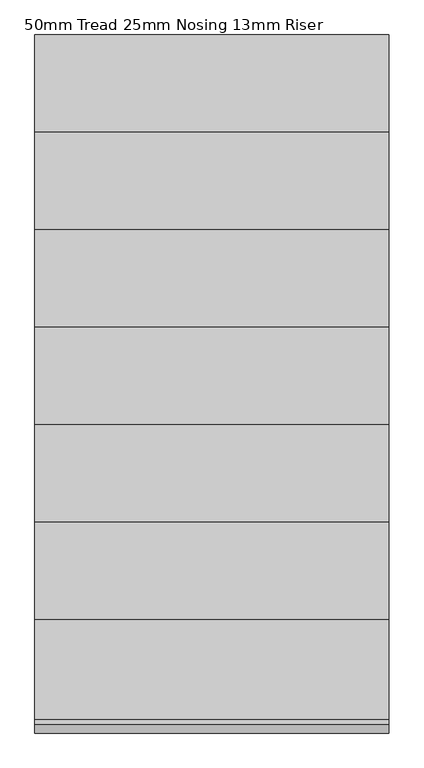
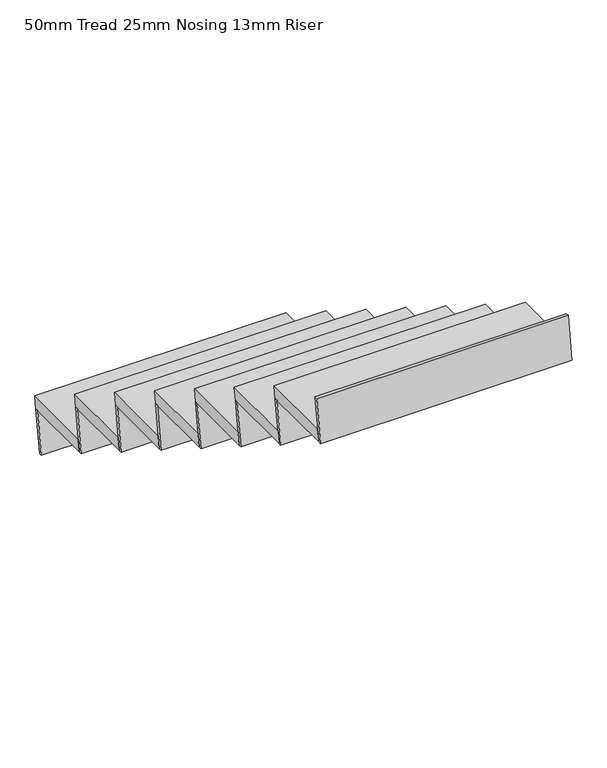
"""IFC4 building model written with IfcOpenShell, lengths in millimetres: stair flight geometry, 50mm Tread 25mm Nosing 13mm Riser."""

from ifc_helpers import new_model, si_unit, frame, origin, place, context, project, spatial, polyline, outline, extrude, source, transform, mapped, element, save


def stair_flight_50mm_tread_25mm_nosing_13mm_riser_d224a7c8(model_context):
    return source(origin(), model_context, "Body", "SweptSolid", [
        extrude(outline(polyline([(9522.57664, 869.5652174), (9822.57664, 869.5652174), (9815.38914, 819.5652174), (9515.38914, 819.5652174), (9522.57664, 869.5652174)])), frame((-8867.5141631, 0.0, 0.0), z_axis=(1.0, 0.0, 0.0), x_axis=(0.0, 1.0, 0.0)), (0.0, 0.0, 1.0), 1000.0257812),
        extrude(outline(polyline([(9815.38914, 819.5652174), (9790.38914, 645.6521739), (9777.76065, 645.6521739), (9802.76065, 819.5652174), (9815.38914, 819.5652174)])), frame((-8867.5141631, 0.0, 0.0), z_axis=(1.0, 0.0, 0.0), x_axis=(0.0, 1.0, 0.0)), (0.0, 0.0, 1.0), 1000.0257812),
        extrude(outline(polyline([(9540.38914, 993.4782609), (9515.38914, 819.5652174), (9502.76065, 819.5652174), (9527.76065, 993.4782609), (9540.38914, 993.4782609)])), frame((-8867.5141631, 0.0, 0.0), z_axis=(1.0, 0.0, 0.0), x_axis=(0.0, 1.0, 0.0)), (0.0, 0.0, 1.0), 1000.0257812),
        extrude(outline(polyline([(9247.57664, 1043.4782609), (9547.57664, 1043.4782609), (9540.38914, 993.4782609), (9240.38914, 993.4782609), (9247.57664, 1043.4782609)])), frame((-8867.5141631, 0.0, 0.0), z_axis=(1.0, 0.0, 0.0), x_axis=(0.0, 1.0, 0.0)), (0.0, 0.0, 1.0), 1000.0257812),
        extrude(outline(polyline([(9265.38914, 1167.3913043), (9240.38914, 993.4782609), (9227.76065, 993.4782609), (9252.76065, 1167.3913043), (9265.38914, 1167.3913043)])), frame((-8867.5141631, 0.0, 0.0), z_axis=(1.0, 0.0, 0.0), x_axis=(0.0, 1.0, 0.0)), (0.0, 0.0, 1.0), 1000.0257812),
        extrude(outline(polyline([(8972.57664, 1217.3913043), (9272.57664, 1217.3913043), (9265.38914, 1167.3913043), (8965.38914, 1167.3913043), (8972.57664, 1217.3913043)])), frame((-8867.5141631, 0.0, 0.0), z_axis=(1.0, 0.0, 0.0), x_axis=(0.0, 1.0, 0.0)), (0.0, 0.0, 1.0), 1000.0257812),
        extrude(outline(polyline([(8990.38914, 1341.3043478), (8965.38914, 1167.3913043), (8952.76065, 1167.3913043), (8977.76065, 1341.3043478), (8990.38914, 1341.3043478)])), frame((-8867.5141631, 0.0, 0.0), z_axis=(1.0, 0.0, 0.0), x_axis=(0.0, 1.0, 0.0)), (0.0, 0.0, 1.0), 1000.0257812),
        extrude(outline(polyline([(8697.57664, 1391.3043478), (8997.57664, 1391.3043478), (8990.38914, 1341.3043478), (8690.38914, 1341.3043478), (8697.57664, 1391.3043478)])), frame((-8867.5141631, 0.0, 0.0), z_axis=(1.0, 0.0, 0.0), x_axis=(0.0, 1.0, 0.0)), (0.0, 0.0, 1.0), 1000.0257812),
        extrude(outline(polyline([(8715.38914, 1515.2173913), (8690.38914, 1341.3043478), (8677.76065, 1341.3043478), (8702.76065, 1515.2173913), (8715.38914, 1515.2173913)])), frame((-8867.5141631, 0.0, 0.0), z_axis=(1.0, 0.0, 0.0), x_axis=(0.0, 1.0, 0.0)), (0.0, 0.0, 1.0), 1000.0257812),
        extrude(outline(polyline([(8422.57664, 1565.2173913), (8722.57664, 1565.2173913), (8715.38914, 1515.2173913), (8415.38914, 1515.2173913), (8422.57664, 1565.2173913)])), frame((-8867.5141631, 0.0, 0.0), z_axis=(1.0, 0.0, 0.0), x_axis=(0.0, 1.0, 0.0)), (0.0, 0.0, 1.0), 1000.0257812),
        extrude(outline(polyline([(8440.38914, 1689.1304348), (8415.38914, 1515.2173913), (8402.76065, 1515.2173913), (8427.76065, 1689.1304348), (8440.38914, 1689.1304348)])), frame((-8867.5141631, 0.0, 0.0), z_axis=(1.0, 0.0, 0.0), x_axis=(0.0, 1.0, 0.0)), (0.0, 0.0, 1.0), 1000.0257812),
        extrude(outline(polyline([(8147.57664, 1739.1304348), (8447.57664, 1739.1304348), (8440.38914, 1689.1304348), (8140.38914, 1689.1304348), (8147.57664, 1739.1304348)])), frame((-8867.5141631, 0.0, 0.0), z_axis=(1.0, 0.0, 0.0), x_axis=(0.0, 1.0, 0.0)), (0.0, 0.0, 1.0), 1000.0257812),
        extrude(outline(polyline([(8165.38914, 1863.0434783), (8140.38914, 1689.1304348), (8127.76065, 1689.1304348), (8152.76065, 1863.0434783), (8165.38914, 1863.0434783)])), frame((-8867.5141631, 0.0, 0.0), z_axis=(1.0, 0.0, 0.0), x_axis=(0.0, 1.0, 0.0)), (0.0, 0.0, 1.0), 1000.0257812),
        extrude(outline(polyline([(7890.38914, 2036.9565217), (7865.38914, 1863.0434783), (7852.76065, 1863.0434783), (7877.76065, 2036.9565217), (7890.38914, 2036.9565217)])), frame((-8867.5141631, 0.0, 0.0), z_axis=(1.0, 0.0, 0.0), x_axis=(0.0, 1.0, 0.0)), (0.0, 0.0, 1.0), 1000.0257812),
        extrude(outline(polyline([(7872.57664, 1913.0434783), (8172.57664, 1913.0434783), (8165.38914, 1863.0434783), (7865.38914, 1863.0434783), (7872.57664, 1913.0434783)])), frame((-8867.5141631, 0.0, 0.0), z_axis=(1.0, 0.0, 0.0), x_axis=(0.0, 1.0, 0.0)), (0.0, 0.0, 1.0), 1000.0257812),
    ])


if __name__ == "__main__":
    model = new_model("IFC4")
    model_context = context("Model", 3, world=origin())
    ifc_project = project(units=[si_unit("LENGTHUNIT", "METRE", prefix="MILLI")], contexts=[model_context])
    site = spatial("IfcSite", under=ifc_project)
    building = spatial("IfcBuilding", under=site)
    placement = place(None, origin())
    stair_flight_50mm_tread_25mm_nosing_13mm_riser_shape = stair_flight_50mm_tread_25mm_nosing_13mm_riser_d224a7c8(model_context)
    element("IfcStairFlight", 1, ObjectType="50mm Tread 25mm Nosing 13mm Riser", at=placement, inside=building, context=model_context, shape_type="MappedRepresentation", body=[
        mapped(stair_flight_50mm_tread_25mm_nosing_13mm_riser_shape, transform((0.0, 0.0, 0.0), x_axis=(1.0, 0.0, 0.0), y_axis=(0.0, 1.0, 0.0), z_axis=(0.0, 0.0, 1.0))),
    ])
    save(model, "model.ifc")
